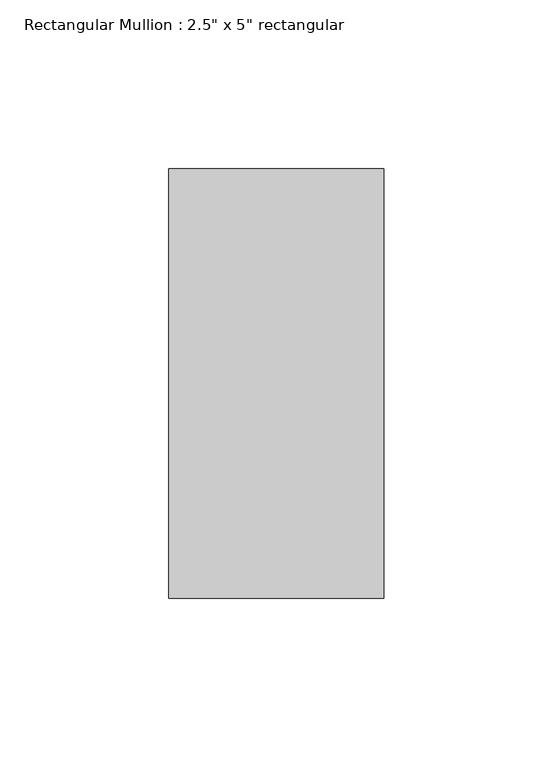
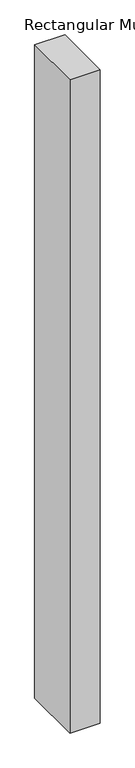
"""IFC4 building model written with IfcOpenShell, lengths in millimetres: member geometry."""

from ifc_helpers import new_model, si_unit, frame, origin, place, context, project, spatial, polyline, outline, extrude, source, transform, mapped, element, save


def member_46c3daae(model_context):
    return source(origin(), model_context, "Body", "SweptSolid", [
        extrude(outline(polyline([(0.0, 63.5), (0.0, -63.5), (-63.5, -63.5), (-63.5, 63.5), (0.0, 63.5)])), frame((0.0, 0.0, -1442.3193903), z_axis=(0.0, 0.0, 1.0), x_axis=(1.0, 0.0, 0.0)), (0.0, 0.0, 1.0), 1442.3193903),
    ])


if __name__ == "__main__":
    model = new_model("IFC4")
    model_context = context("Model", 3, world=origin())
    ifc_project = project(units=[si_unit("LENGTHUNIT", "METRE", prefix="MILLI")], contexts=[model_context])
    site = spatial("IfcSite", under=ifc_project)
    building = spatial("IfcBuilding", under=site)
    placement = place(None, origin())
    member_shape = member_46c3daae(model_context)
    element("IfcMember", 1, ObjectType="Rectangular Mullion : 2.5\" x 5\" rectangular", at=placement, inside=building, context=model_context, shape_type="MappedRepresentation", body=[
        mapped(member_shape, transform((0.0, 0.0, 0.0), x_axis=(1.0, 0.0, 0.0), y_axis=(0.0, 1.0, 0.0), z_axis=(0.0, 0.0, 1.0))),
    ])
    save(model, "model.ifc")

# Revit data of these elements
# Type "Rectangular Mullion : 2.5\" x 5\" rectangular"
#   built-in parameter 1007304 = 0.416667 (stored number, unit not read)
#   built-in parameter 1007301 = 0.104167 (stored number, unit not read)
#   built-in parameter 1007300 = 0.104167 (stored number, unit not read)
# Element 1 (IfcMember, "Rectangular Mullion : 2.5\" x 5\" rectangular")
#   Materials on its faces: "Aluminum"
# Materials
#   "Aluminum": class "Metal", colour RGB 247 247 247, transparency 0, Description = "Aluminum 6061", Cost = 0
